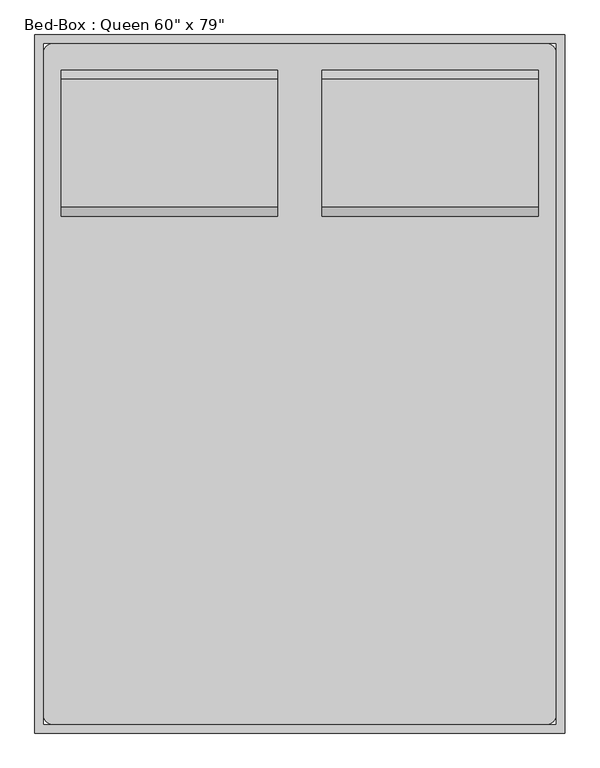
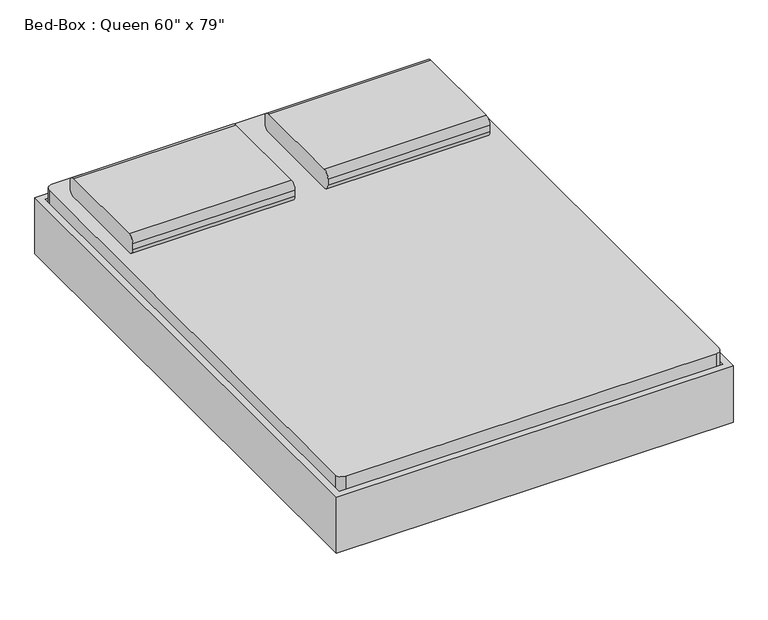
"""IFC4 building model written with IfcOpenShell, lengths in millimetres: furniture geometry."""

from ifc_helpers import new_model, si_unit, point, frame, frame_2d, origin, place, context, project, spatial, polyline, circle_curve, trimmed, segment, composite_curve, outline, extrude, source, transform, mapped, element, save
from ifc_brep_helpers import plane_surface, cylinder_surface, revolved_surface, advanced_brep


def furniture_0315470b(model_context):
    return source(origin(), model_context, "Body", "SolidModel", [
        advanced_brep(
        [(-397.447541, -932.9295082, 196.85), (-397.447541, -932.9295082, 177.8), (-397.447541, -1009.1295082, 177.8), (-397.447541, -1009.1295082, 196.85), (-334.5113525, -932.9295082, 196.85), (-346.647541, -932.9295082, 177.8), (-346.647541, -1009.1295082, 177.8), (-334.5113525, -1009.1295082, 196.85), (-253.3115092, -932.9295082, 22.716374), (-270.5766725, -932.9295082, 14.6654962), (-270.5766725, -1009.1295082, 14.6654962), (-253.3115092, -1009.1295082, 22.716374), (-247.5564547, -932.9295082, 0.0), (-247.5564547, -932.9295082, 19.05), (-247.5564547, -1009.1295082, 0.0), (-247.5564547, -1009.1295082, 19.05), (-168.9439489, -932.9295082, 19.05), (-168.9439489, -932.9295082, 0.0), (-168.9439489, -1009.1295082, 0.0), (-168.9439489, -1009.1295082, 19.05), (-156.2439489, -932.9295082, 3.4029547), (-165.7689489, -932.9295082, 19.9007387), (-156.2439489, -1009.1295082, 3.4029547), (-165.7689489, -1009.1295082, 19.9007387), (-101.2513357, -932.9295082, 57.15), (-96.1469036, -932.9295082, 38.1), (-96.1469036, -1009.1295082, 38.1), (-101.2513357, -1009.1295082, 57.15), (779.5562537, -932.9295082, 57.15), (774.4518216, -932.9295082, 38.1), (774.4518216, -1009.1295082, 38.1), (779.5562537, -1009.1295082, 57.15), (844.0738669, -932.9295082, 19.9007387), (834.5488669, -932.9295082, 3.4029547), (834.5488669, -1009.1295082, 3.4029547), (844.0738669, -1009.1295082, 19.9007387), (847.2488669, -932.9295082, 0.0), (847.2488669, -932.9295082, 19.05), (847.2488669, -1009.1295082, 0.0), (847.2488669, -1009.1295082, 19.05), (925.8613728, -932.9295082, 19.05), (925.8613728, -932.9295082, 0.0), (925.8613728, -1009.1295082, 0.0), (925.8613728, -1009.1295082, 19.05), (948.8815906, -932.9295082, 14.6654962), (931.6164272, -932.9295082, 22.716374), (948.8815906, -1009.1295082, 14.6654962), (931.6164272, -1009.1295082, 22.716374), (1012.8162705, -932.9295082, 196.85), (1024.952459, -932.9295082, 177.8), (1024.952459, -1009.1295082, 177.8), (1012.8162705, -1009.1295082, 196.85), (1075.752459, -932.9295082, 196.85), (1075.752459, -1009.1295082, 196.85), (1075.752459, -1009.1295082, 177.8), (1075.752459, -932.9295082, 177.8)],
        [
            (0, 1),
            (1, 2),
            (2, 3),
            (3, 0),
            (0, 4),
            (4, 5),
            (5, 1),
            (5, 6),
            (6, 2),
            (6, 7),
            (7, 3),
            (7, 4),
            (4, 8),
            (8, 9),
            (9, 5),
            (9, 10),
            (10, 6),
            (10, 11),
            (11, 7),
            (11, 8),
            (12, 9, circle_curve(frame((-247.5564547, -932.9295082, 25.4), z_axis=(0.0, 1.0, 0.0), x_axis=(-0.906307787036663, 0.0, -0.4226182617406713)), 25.4)),
            (8, 13, circle_curve(frame((-247.5564547, -932.9295082, 25.4), z_axis=(0.0, -1.0, 0.0), x_axis=(-0.906307787036663, 0.0, -0.4226182617406713)), 6.35)),
            (13, 12),
            (14, 10, circle_curve(frame((-247.5564547, -1009.1295082, 25.4), z_axis=(0.0, 1.0, 0.0), x_axis=(-0.906307787036663, 0.0, -0.4226182617406713)), 25.4)),
            (12, 14),
            (15, 11, circle_curve(frame((-247.5564547, -1009.1295082, 25.4), z_axis=(0.0, 1.0, 0.0), x_axis=(-0.906307787036663, 0.0, -0.4226182617406713)), 6.35)),
            (14, 15),
            (15, 13),
            (13, 16),
            (16, 17),
            (17, 12),
            (17, 18),
            (18, 14),
            (18, 19),
            (19, 15),
            (19, 16),
            (20, 17, circle_curve(frame((-168.9439489, -932.9295082, 25.4), z_axis=(0.0, 1.0, 0.0), x_axis=(0.0, 0.0, -1.0)), 25.4)),
            (16, 21, circle_curve(frame((-168.9439489, -932.9295082, 25.4), z_axis=(0.0, -1.0, 0.0), x_axis=(0.0, 0.0, -1.0)), 6.35)),
            (21, 20),
            (22, 18, circle_curve(frame((-168.9439489, -1009.1295082, 25.4), z_axis=(0.0, 1.0, 0.0), x_axis=(0.0, 0.0, -1.0)), 25.4)),
            (20, 22),
            (23, 19, circle_curve(frame((-168.9439489, -1009.1295082, 25.4), z_axis=(0.0, 1.0, 0.0), x_axis=(0.0, 0.0, -1.0)), 6.35)),
            (22, 23),
            (23, 21),
            (21, 24),
            (24, 25),
            (25, 20),
            (25, 26),
            (26, 22),
            (26, 27),
            (27, 23),
            (27, 24),
            (24, 28),
            (28, 29),
            (29, 25),
            (29, 30),
            (30, 26),
            (30, 31),
            (31, 27),
            (31, 28),
            (28, 32),
            (32, 33),
            (33, 29),
            (33, 34),
            (34, 30),
            (34, 35),
            (35, 31),
            (35, 32),
            (36, 33, circle_curve(frame((847.2488669, -932.9295082, 25.4), z_axis=(0.0, 1.0, 0.0), x_axis=(-0.5000000000000479, 0.0, -0.866025403784411)), 25.4)),
            (32, 37, circle_curve(frame((847.2488669, -932.9295082, 25.4), z_axis=(0.0, -1.0, 0.0), x_axis=(-0.5000000000000479, 0.0, -0.866025403784411)), 6.35)),
            (37, 36),
            (38, 34, circle_curve(frame((847.2488669, -1009.1295082, 25.4), z_axis=(0.0, 1.0, 0.0), x_axis=(-0.5000000000000479, 0.0, -0.866025403784411)), 25.4)),
            (36, 38),
            (39, 35, circle_curve(frame((847.2488669, -1009.1295082, 25.4), z_axis=(0.0, 1.0, 0.0), x_axis=(-0.5000000000000479, 0.0, -0.866025403784411)), 6.35)),
            (38, 39),
            (39, 37),
            (37, 40),
            (40, 41),
            (41, 36),
            (41, 42),
            (42, 38),
            (42, 43),
            (43, 39),
            (43, 40),
            (44, 41, circle_curve(frame((925.8613728, -932.9295082, 25.4), z_axis=(0.0, 1.0, 0.0), x_axis=(0.0, 0.0, -1.0)), 25.4)),
            (40, 45, circle_curve(frame((925.8613728, -932.9295082, 25.4), z_axis=(0.0, -1.0, 0.0), x_axis=(0.0, 0.0, -1.0)), 6.35)),
            (45, 44),
            (46, 42, circle_curve(frame((925.8613728, -1009.1295082, 25.4), z_axis=(0.0, 1.0, 0.0), x_axis=(0.0, 0.0, -1.0)), 25.4)),
            (44, 46),
            (47, 43, circle_curve(frame((925.8613728, -1009.1295082, 25.4), z_axis=(0.0, 1.0, 0.0), x_axis=(0.0, 0.0, -1.0)), 6.35)),
            (46, 47),
            (47, 45),
            (45, 48),
            (48, 49),
            (49, 44),
            (49, 50),
            (50, 46),
            (50, 51),
            (51, 47),
            (51, 48),
            (52, 53),
            (53, 54),
            (54, 55),
            (55, 52),
            (48, 52),
            (55, 49),
            (54, 50),
            (53, 51),
        ],
        [
            plane_surface(frame((-397.447541, -1237.7295082, -127.5947323), z_axis=(-1.0, 0.0, 0.0), x_axis=(0.0, 1.0, 0.0))),
            plane_surface(frame((-397.447541, -932.9295082, 196.85), z_axis=(0.0, 1.0, 0.0), x_axis=(1.0, 0.0, 0.0))),
            plane_surface(frame((-397.447541, -932.9295082, 177.8), z_axis=(0.0, 0.0, -1.0), x_axis=(1.0, 0.0, 0.0))),
            plane_surface(frame((-397.447541, -1009.1295082, 177.8), z_axis=(0.0, -1.0, 0.0), x_axis=(1.0, 0.0, 0.0))),
            plane_surface(frame((-397.447541, -1009.1295082, 196.85), z_axis=(0.0, 0.0, 1.0), x_axis=(1.0, 0.0, 0.0))),
            plane_surface(frame((-334.5113525, -932.9295082, 196.85), z_axis=(0.0, 1.0, 0.0), x_axis=(0.4226182617406707, 0.0, -0.9063077870366634))),
            plane_surface(frame((-346.647541, -932.9295082, 177.8), z_axis=(-0.9063077870366635, 0.0, -0.4226182617406707), x_axis=(0.4226182617406707, 0.0, -0.9063077870366635))),
            plane_surface(frame((-346.647541, -1009.1295082, 177.8), z_axis=(0.0, -1.0, 0.0), x_axis=(0.422618261740671, 0.0, -0.9063077870366633))),
            plane_surface(frame((-334.5113525, -1009.1295082, 196.85), z_axis=(0.9063077870366633, 0.0, 0.42261826174067113), x_axis=(0.42261826174067113, 0.0, -0.9063077870366633))),
            plane_surface(frame((-247.5564547, -932.9295082, 25.4), z_axis=(0.0, 1.0, 0.0), x_axis=(-0.906307787036663, 0.0, -0.4226182617406713))),
            cylinder_surface(frame((-247.5564547, -1237.7295082, 25.4), z_axis=(0.0, -1.0, 0.0), x_axis=(-0.906307787036663, 0.0, -0.4226182617406713)), 25.4),
            plane_surface(frame((-247.5564547, -1009.1295082, 25.4), z_axis=(0.0, -1.0, 0.0), x_axis=(-0.906307787036663, 0.0, -0.4226182617406713))),
            revolved_surface(polyline([(-253.3115091476828, -1009.1295082, 22.716374037946736), (-253.3115091476828, -932.9295082, 22.716374037946736)]), (-247.5564547, -1237.7295082, 25.4), (0.0, -1.0, 0.0)),
            plane_surface(frame((-247.5564547, -932.9295082, 19.05), z_axis=(0.0, 1.0, 0.0), x_axis=(1.0, 0.0, 0.0))),
            plane_surface(frame((-247.5564547, -932.9295082, 0.0), z_axis=(0.0, 0.0, -1.0), x_axis=(1.0, 0.0, 0.0))),
            plane_surface(frame((-247.5564547, -1009.1295082, 0.0), z_axis=(0.0, -1.0, 0.0), x_axis=(1.0, 0.0, 0.0))),
            plane_surface(frame((-247.5564547, -1009.1295082, 19.05), z_axis=(0.0, 0.0, 1.0), x_axis=(1.0, 0.0, 0.0))),
            plane_surface(frame((-168.9439489, -932.9295082, 25.4), z_axis=(0.0, 1.0, 0.0), x_axis=(0.0, 0.0, -1.0))),
            cylinder_surface(frame((-168.9439489, -1237.7295082, 25.4), z_axis=(0.0, -1.0, 0.0), x_axis=(0.0, 0.0, -1.0)), 25.4),
            plane_surface(frame((-168.9439489, -1009.1295082, 25.4), z_axis=(0.0, -1.0, 0.0), x_axis=(0.0, 0.0, -1.0))),
            revolved_surface(polyline([(-168.9439489, -1009.1295082, 19.049999999999997), (-168.9439489, -932.9295082, 19.049999999999997)]), (-168.9439489, -1237.7295082, 25.4), (0.0, -1.0, 0.0)),
            plane_surface(frame((-165.7689489, -932.9295082, 19.9007387), z_axis=(0.0, 1.0, 0.0), x_axis=(0.8660254037844788, 0.0, 0.4999999999999306))),
            plane_surface(frame((-156.2439489, -932.9295082, 3.4029547), z_axis=(0.49999999999993017, 0.0, -0.866025403784479), x_axis=(0.866025403784479, 0.0, 0.49999999999993017))),
            plane_surface(frame((-156.2439489, -1009.1295082, 3.4029547), z_axis=(0.0, -1.0, 0.0), x_axis=(0.8660254037844785, 0.0, 0.49999999999993106))),
            plane_surface(frame((-165.7689489, -1009.1295082, 19.9007387), z_axis=(-0.4999999999999309, 0.0, 0.8660254037844786), x_axis=(0.8660254037844786, 0.0, 0.4999999999999309))),
            plane_surface(frame((-101.2513357, -932.9295082, 57.15), z_axis=(0.0, 1.0, 0.0), x_axis=(1.0, 0.0, 0.0))),
            plane_surface(frame((-96.1469036, -932.9295082, 38.1), z_axis=(0.0, 0.0, -1.0), x_axis=(1.0, 0.0, 0.0))),
            plane_surface(frame((-96.1469036, -1009.1295082, 38.1), z_axis=(0.0, -1.0, 0.0), x_axis=(1.0, 0.0, 0.0))),
            plane_surface(frame((-101.2513357, -1009.1295082, 57.15), z_axis=(0.0, 0.0, 1.0), x_axis=(1.0, 0.0, 0.0))),
            plane_surface(frame((779.5562537, -932.9295082, 57.15), z_axis=(0.0, 1.0000000000000002, 0.0), x_axis=(0.8660254037844106, 0.0, -0.5000000000000487))),
            plane_surface(frame((774.4518216, -932.9295082, 38.1), z_axis=(-0.5000000000000477, 0.0, -0.8660254037844112), x_axis=(0.8660254037844112, 0.0, -0.5000000000000477))),
            plane_surface(frame((774.4518216, -1009.1295082, 38.1), z_axis=(0.0, -1.0000000000000002, 0.0), x_axis=(0.8660254037844105, 0.0, -0.500000000000049))),
            plane_surface(frame((779.5562537, -1009.1295082, 57.15), z_axis=(0.5000000000000498, 0.0, 0.8660254037844098), x_axis=(0.8660254037844098, 0.0, -0.5000000000000498))),
            plane_surface(frame((847.2488669, -932.9295082, 25.4), z_axis=(0.0, 1.0000000000000002, 0.0), x_axis=(-0.500000000000048, 0.0, -0.8660254037844111))),
            cylinder_surface(frame((847.2488669, -1237.7295082, 25.4), z_axis=(0.0, -1.0, 0.0), x_axis=(-0.5000000000000479, 0.0, -0.866025403784411)), 25.4),
            plane_surface(frame((847.2488669, -1009.1295082, 25.4), z_axis=(0.0, -1.0000000000000002, 0.0), x_axis=(-0.500000000000048, 0.0, -0.8660254037844111))),
            revolved_surface(polyline([(844.0738668999998, -1009.1295082, 19.90073868596899), (844.0738668999998, -932.9295082, 19.90073868596899)]), (847.2488669, -1237.7295082, 25.4), (0.0, -1.0, 0.0)),
            plane_surface(frame((847.2488669, -932.9295082, 19.05), z_axis=(0.0, 1.0, 0.0), x_axis=(1.0, 0.0, 0.0))),
            plane_surface(frame((847.2488669, -932.9295082, 0.0), z_axis=(0.0, 0.0, -1.0), x_axis=(1.0, 0.0, 0.0))),
            plane_surface(frame((847.2488669, -1009.1295082, 0.0), z_axis=(0.0, -1.0, 0.0), x_axis=(1.0, 0.0, 0.0))),
            plane_surface(frame((847.2488669, -1009.1295082, 19.05), z_axis=(0.0, 0.0, 1.0), x_axis=(1.0, 0.0, 0.0))),
            plane_surface(frame((925.8613728, -932.9295082, 25.4), z_axis=(0.0, 1.0, 0.0), x_axis=(0.0, 0.0, -1.0))),
            cylinder_surface(frame((925.8613728, -1237.7295082, 25.4), z_axis=(0.0, -1.0, 0.0), x_axis=(0.0, 0.0, -1.0)), 25.4),
            plane_surface(frame((925.8613728, -1009.1295082, 25.4), z_axis=(0.0, -1.0, 0.0), x_axis=(0.0, 0.0, -1.0))),
            revolved_surface(polyline([(925.8613728, -1009.1295082, 19.049999999999997), (925.8613728, -932.9295082, 19.049999999999997)]), (925.8613728, -1237.7295082, 25.4), (0.0, -1.0, 0.0)),
            plane_surface(frame((931.6164272, -932.9295082, 22.716374), z_axis=(0.0, 1.0, 0.0), x_axis=(0.4226182617405411, 0.0, 0.9063077870367238))),
            plane_surface(frame((948.8815906, -932.9295082, 14.6654962), z_axis=(0.9063077870367237, 0.0, -0.4226182617405414), x_axis=(0.4226182617405414, 0.0, 0.9063077870367237))),
            plane_surface(frame((948.8815906, -1009.1295082, 14.6654962), z_axis=(0.0, -1.0, 0.0), x_axis=(0.42261826174054123, 0.0, 0.9063077870367238))),
            plane_surface(frame((931.6164272, -1009.1295082, 22.716374), z_axis=(-0.9063077870367237, 0.0, 0.4226182617405414), x_axis=(0.4226182617405414, 0.0, 0.9063077870367237))),
            plane_surface(frame((1075.752459, -1237.7295082, -127.5947323), z_axis=(1.0, 0.0, 0.0), x_axis=(0.0, 1.0, 0.0))),
            plane_surface(frame((1012.8162705, -932.9295082, 196.85), z_axis=(0.0, 1.0, 0.0), x_axis=(1.0, 0.0, 0.0))),
            plane_surface(frame((1024.952459, -932.9295082, 177.8), z_axis=(0.0, 0.0, -1.0), x_axis=(1.0, 0.0, 0.0))),
            plane_surface(frame((1024.952459, -1009.1295082, 177.8), z_axis=(0.0, -1.0, 0.0), x_axis=(1.0, 0.0, 0.0))),
            plane_surface(frame((1012.8162705, -1009.1295082, 196.85), z_axis=(0.0, 0.0, 1.0), x_axis=(1.0, 0.0, 0.0))),
        ],
        [
            (0, [[1, 2, 3, 4]]),
            (1, [[-1, 5, 6, 7]]),
            (2, [[-2, -7, 8, 9]]),
            (3, [[-3, -9, 10, 11]]),
            (4, [[-4, -11, 12, -5]]),
            (5, [[-6, 13, 14, 15]]),
            (6, [[-8, -15, 16, 17]]),
            (7, [[-10, -17, 18, 19]]),
            (8, [[-12, -19, 20, -13]]),
            (9, [[21, -14, 22, 23]]),
            (10, [[24, -16, -21, 25]]),
            (11, [[26, -18, -24, 27]]),
            (12, [[-22, -20, -26, 28]]),
            (13, [[-23, 29, 30, 31]]),
            (14, [[-25, -31, 32, 33]]),
            (15, [[-27, -33, 34, 35]]),
            (16, [[-28, -35, 36, -29]]),
            (17, [[37, -30, 38, 39]]),
            (18, [[40, -32, -37, 41]]),
            (19, [[42, -34, -40, 43]]),
            (20, [[-38, -36, -42, 44]]),
            (21, [[-39, 45, 46, 47]]),
            (22, [[-41, -47, 48, 49]]),
            (23, [[-43, -49, 50, 51]]),
            (24, [[-44, -51, 52, -45]]),
            (25, [[-46, 53, 54, 55]]),
            (26, [[-48, -55, 56, 57]]),
            (27, [[-50, -57, 58, 59]]),
            (28, [[-52, -59, 60, -53]]),
            (29, [[-54, 61, 62, 63]]),
            (30, [[-56, -63, 64, 65]]),
            (31, [[-58, -65, 66, 67]]),
            (32, [[-60, -67, 68, -61]]),
            (33, [[69, -62, 70, 71]]),
            (34, [[72, -64, -69, 73]]),
            (35, [[74, -66, -72, 75]]),
            (36, [[-70, -68, -74, 76]]),
            (37, [[-71, 77, 78, 79]]),
            (38, [[-73, -79, 80, 81]]),
            (39, [[-75, -81, 82, 83]]),
            (40, [[-76, -83, 84, -77]]),
            (41, [[85, -78, 86, 87]]),
            (42, [[88, -80, -85, 89]]),
            (43, [[90, -82, -88, 91]]),
            (44, [[-86, -84, -90, 92]]),
            (45, [[-87, 93, 94, 95]]),
            (46, [[-89, -95, 96, 97]]),
            (47, [[-91, -97, 98, 99]]),
            (48, [[-92, -99, 100, -93]]),
            (49, [[101, 102, 103, 104]]),
            (50, [[-94, 105, -104, 106]]),
            (51, [[-96, -106, -103, 107]]),
            (52, [[-98, -107, -102, 108]]),
            (53, [[-100, -108, -101, -105]]),
        ],
    ),
        extrude(outline(composite_curve([segment(polyline([(-372.047541, 743.4704918), (1050.352459, 743.4704918)]), True, "CONTINUOUS"), segment(trimmed(circle_curve(frame_2d((1050.352459, 718.0704918)), 25.4), [point((1050.352459, 743.4704918))], [point((1075.752459, 718.0704918))], False, "CARTESIAN"), True, "CONTINUOUS"), segment(polyline([(1075.752459, 718.0704918), (1075.752459, -1186.9295082)]), True, "CONTINUOUS"), segment(trimmed(circle_curve(frame_2d((1050.352459, -1186.9295082)), 25.4), [point((1075.752459, -1186.9295082))], [point((1050.352459, -1212.3295082))], False, "CARTESIAN"), True, "CONTINUOUS"), segment(polyline([(1050.352459, -1212.3295082), (-372.047541, -1212.3295082)]), True, "CONTINUOUS"), segment(trimmed(circle_curve(frame_2d((-372.047541, -1186.9295082)), 25.4), [point((-372.047541, -1212.3295082))], [point((-397.447541, -1186.9295082))], False, "CARTESIAN"), True, "CONTINUOUS"), segment(polyline([(-397.447541, -1186.9295082), (-397.447541, 718.0704918)]), True, "CONTINUOUS"), segment(trimmed(circle_curve(frame_2d((-372.047541, 718.0704918)), 25.4), [point((-397.447541, 718.0704918))], [point((-372.047541, 743.4704918))], False, "CARTESIAN"), True, "CONTINUOUS")], self_intersect=False)), frame((0.0, 0.0, 203.2), z_axis=(0.0, 0.0, 1.0), x_axis=(1.0, 0.0, 0.0)), (0.0, 0.0, 1.0), 203.2),
        advanced_brep(
        [(-397.1231784, 514.8704918, 177.8), (-397.1231784, 438.6704918, 177.8), (-397.1231784, 438.6704918, 196.85), (-397.1231784, 514.8704918, 196.85), (-346.3231784, 514.8704918, 177.8), (-346.3231784, 438.6704918, 177.8), (-334.1869899, 438.6704918, 196.85), (-334.1869899, 514.8704918, 196.85), (-270.2523099, 514.8704918, 14.6654962), (-270.2523099, 438.6704918, 14.6654962), (-252.9871466, 438.6704918, 22.716374), (-252.9871466, 514.8704918, 22.716374), (-247.2320921, 438.6704918, 0.0), (-247.2320921, 514.8704918, 0.0), (-247.2320921, 438.6704918, 19.05), (-247.2320921, 514.8704918, 19.05), (-168.6195862, 514.8704918, 0.0), (-168.6195862, 438.6704918, 0.0), (-168.6195862, 438.6704918, 19.05), (-168.6195862, 514.8704918, 19.05), (-155.9195862, 438.6704918, 3.4029547), (-155.9195862, 514.8704918, 3.4029547), (-165.4445862, 438.6704918, 19.9007387), (-165.4445862, 514.8704918, 19.9007387), (-95.822541, 514.8704918, 38.1), (-95.822541, 438.6704918, 38.1), (-100.9269731, 438.6704918, 57.15), (-100.9269731, 514.8704918, 57.15), (774.4518216, 514.8704918, 38.1), (774.4518216, 438.6704918, 38.1), (779.5562537, 438.6704918, 57.15), (779.5562537, 514.8704918, 57.15), (834.5488669, 514.8704918, 3.4029547), (834.5488669, 438.6704918, 3.4029547), (844.0738669, 438.6704918, 19.9007387), (844.0738669, 514.8704918, 19.9007387), (847.2488669, 438.6704918, 0.0), (847.2488669, 514.8704918, 0.0), (847.2488669, 438.6704918, 19.05), (847.2488669, 514.8704918, 19.05), (925.8613728, 514.8704918, 0.0), (925.8613728, 438.6704918, 0.0), (925.8613728, 438.6704918, 19.05), (925.8613728, 514.8704918, 19.05), (948.8815906, 438.6704918, 14.6654962), (948.8815906, 514.8704918, 14.6654962), (931.6164272, 438.6704918, 22.716374), (931.6164272, 514.8704918, 22.716374), (1024.952459, 514.8704918, 177.8), (1024.952459, 438.6704918, 177.8), (1012.8162705, 438.6704918, 196.85), (1012.8162705, 514.8704918, 196.85), (1075.752459, 514.8704918, 177.8), (1075.752459, 514.8704918, 196.85), (1075.752459, 438.6704918, 196.85), (1075.752459, 438.6704918, 177.8)],
        [
            (0, 1),
            (1, 2),
            (2, 3),
            (3, 0),
            (0, 4),
            (4, 5),
            (5, 1),
            (5, 6),
            (6, 2),
            (6, 7),
            (7, 3),
            (7, 4),
            (4, 8),
            (8, 9),
            (9, 5),
            (9, 10),
            (10, 6),
            (10, 11),
            (11, 7),
            (11, 8),
            (12, 9, circle_curve(frame((-247.2320921, 438.6704918, 25.4), z_axis=(0.0, 1.0, 0.0), x_axis=(-0.9063077870366486, 0.0, -0.42261826174070233)), 25.4)),
            (8, 13, circle_curve(frame((-247.2320921, 514.8704918, 25.4), z_axis=(0.0, -1.0, 0.0), x_axis=(-0.9063077870366486, 0.0, -0.42261826174070233)), 25.4)),
            (13, 12),
            (14, 10, circle_curve(frame((-247.2320921, 438.6704918, 25.4), z_axis=(0.0, 1.0, 0.0), x_axis=(-0.9063077870366486, 0.0, -0.42261826174070233)), 6.35)),
            (12, 14),
            (15, 11, circle_curve(frame((-247.2320921, 514.8704918, 25.4), z_axis=(0.0, 1.0, 0.0), x_axis=(-0.9063077870366486, 0.0, -0.42261826174070233)), 6.35)),
            (14, 15),
            (15, 13),
            (13, 16),
            (16, 17),
            (17, 12),
            (17, 18),
            (18, 14),
            (18, 19),
            (19, 15),
            (19, 16),
            (20, 17, circle_curve(frame((-168.6195862, 438.6704918, 25.4), z_axis=(0.0, 1.0, 0.0), x_axis=(0.0, 0.0, -1.0)), 25.4)),
            (16, 21, circle_curve(frame((-168.6195862, 514.8704918, 25.4), z_axis=(0.0, -1.0, 0.0), x_axis=(0.0, 0.0, -1.0)), 25.4)),
            (21, 20),
            (22, 18, circle_curve(frame((-168.6195862, 438.6704918, 25.4), z_axis=(0.0, 1.0, 0.0), x_axis=(0.0, 0.0, -1.0)), 6.35)),
            (20, 22),
            (23, 19, circle_curve(frame((-168.6195862, 514.8704918, 25.4), z_axis=(0.0, 1.0, 0.0), x_axis=(0.0, 0.0, -1.0)), 6.35)),
            (22, 23),
            (23, 21),
            (21, 24),
            (24, 25),
            (25, 20),
            (25, 26),
            (26, 22),
            (26, 27),
            (27, 23),
            (27, 24),
            (24, 28),
            (28, 29),
            (29, 25),
            (29, 30),
            (30, 26),
            (30, 31),
            (31, 27),
            (31, 28),
            (28, 32),
            (32, 33),
            (33, 29),
            (33, 34),
            (34, 30),
            (34, 35),
            (35, 31),
            (35, 32),
            (36, 33, circle_curve(frame((847.2488669, 438.6704918, 25.4), z_axis=(0.0, 1.0, 0.0), x_axis=(-0.5000000000000463, 0.0, -0.8660254037844118)), 25.4)),
            (32, 37, circle_curve(frame((847.2488669, 514.8704918, 25.4), z_axis=(0.0, -1.0, 0.0), x_axis=(-0.5000000000000463, 0.0, -0.8660254037844118)), 25.4)),
            (37, 36),
            (38, 34, circle_curve(frame((847.2488669, 438.6704918, 25.4), z_axis=(0.0, 1.0, 0.0), x_axis=(-0.5000000000000463, 0.0, -0.8660254037844118)), 6.35)),
            (36, 38),
            (39, 35, circle_curve(frame((847.2488669, 514.8704918, 25.4), z_axis=(0.0, 1.0, 0.0), x_axis=(-0.5000000000000463, 0.0, -0.8660254037844118)), 6.35)),
            (38, 39),
            (39, 37),
            (37, 40),
            (40, 41),
            (41, 36),
            (41, 42),
            (42, 38),
            (42, 43),
            (43, 39),
            (43, 40),
            (44, 41, circle_curve(frame((925.8613728, 438.6704918, 25.4), z_axis=(0.0, 1.0, 0.0), x_axis=(0.0, 0.0, -1.0)), 25.4)),
            (40, 45, circle_curve(frame((925.8613728, 514.8704918, 25.4), z_axis=(0.0, -1.0, 0.0), x_axis=(0.0, 0.0, -1.0)), 25.4)),
            (45, 44),
            (46, 42, circle_curve(frame((925.8613728, 438.6704918, 25.4), z_axis=(0.0, 1.0, 0.0), x_axis=(0.0, 0.0, -1.0)), 6.35)),
            (44, 46),
            (47, 43, circle_curve(frame((925.8613728, 514.8704918, 25.4), z_axis=(0.0, 1.0, 0.0), x_axis=(0.0, 0.0, -1.0)), 6.35)),
            (46, 47),
            (47, 45),
            (45, 48),
            (48, 49),
            (49, 44),
            (49, 50),
            (50, 46),
            (50, 51),
            (51, 47),
            (51, 48),
            (52, 53),
            (53, 54),
            (54, 55),
            (55, 52),
            (48, 52),
            (55, 49),
            (54, 50),
            (53, 51),
        ],
        [
            plane_surface(frame((-397.1231784, 768.8704918, -152.9490627), z_axis=(-1.0, 0.0, 0.0), x_axis=(0.0, 1.0, 0.0))),
            plane_surface(frame((-397.1231784, 514.8704918, 177.8), z_axis=(0.0, 0.0, -1.0), x_axis=(1.0, 0.0, 0.0))),
            plane_surface(frame((-397.1231784, 438.6704918, 177.8), z_axis=(0.0, -1.0, 0.0), x_axis=(1.0, 0.0, 0.0))),
            plane_surface(frame((-397.1231784, 438.6704918, 196.85), z_axis=(0.0, 0.0, 1.0), x_axis=(1.0, 0.0, 0.0))),
            plane_surface(frame((-397.1231784, 514.8704918, 196.85), z_axis=(0.0, 1.0, 0.0), x_axis=(1.0, 0.0, 0.0))),
            plane_surface(frame((-346.3231784, 514.8704918, 177.8), z_axis=(-0.9063077870366485, 0.0, -0.4226182617407027), x_axis=(0.4226182617407027, 0.0, -0.9063077870366485))),
            plane_surface(frame((-346.3231784, 438.6704918, 177.8), z_axis=(0.0, -1.0, 0.0), x_axis=(0.4226182617407025, 0.0, -0.9063077870366486))),
            plane_surface(frame((-334.1869899, 438.6704918, 196.85), z_axis=(0.9063077870366484, 0.0, 0.4226182617407028), x_axis=(0.4226182617407028, 0.0, -0.9063077870366484))),
            plane_surface(frame((-334.1869899, 514.8704918, 196.85), z_axis=(0.0, 1.0, 0.0), x_axis=(0.42261826174070277, 0.0, -0.9063077870366485))),
            cylinder_surface(frame((-247.2320921, 768.8704918, 25.4), z_axis=(0.0, -1.0, 0.0), x_axis=(-0.9063077870366486, 0.0, -0.42261826174070233)), 25.4),
            plane_surface(frame((-247.2320921, 438.6704918, 25.4), z_axis=(0.0, -1.0, 0.0), x_axis=(-0.9063077870366486, 0.0, -0.42261826174070233))),
            revolved_surface(polyline([(-252.9871465476827, 438.6704918, 22.71637403794654), (-252.9871465476827, 514.8704918, 22.71637403794654)]), (-247.2320921, 768.8704918, 25.4), (0.0, -1.0, 0.0)),
            plane_surface(frame((-247.2320921, 514.8704918, 25.4), z_axis=(0.0, 1.0, 0.0), x_axis=(-0.9063077870366486, 0.0, -0.42261826174070233))),
            plane_surface(frame((-247.2320921, 514.8704918, 0.0), z_axis=(0.0, 0.0, -1.0), x_axis=(1.0, 0.0, 0.0))),
            plane_surface(frame((-247.2320921, 438.6704918, 0.0), z_axis=(0.0, -1.0, 0.0), x_axis=(1.0, 0.0, 0.0))),
            plane_surface(frame((-247.2320921, 438.6704918, 19.05), z_axis=(0.0, 0.0, 1.0), x_axis=(1.0, 0.0, 0.0))),
            plane_surface(frame((-247.2320921, 514.8704918, 19.05), z_axis=(0.0, 1.0, 0.0), x_axis=(1.0, 0.0, 0.0))),
            cylinder_surface(frame((-168.6195862, 768.8704918, 25.4), z_axis=(0.0, -1.0, 0.0), x_axis=(0.0, 0.0, -1.0)), 25.4),
            plane_surface(frame((-168.6195862, 438.6704918, 25.4), z_axis=(0.0, -1.0, 0.0), x_axis=(0.0, 0.0, -1.0))),
            revolved_surface(polyline([(-168.6195862, 438.6704918, 19.049999999999997), (-168.6195862, 514.8704918, 19.049999999999997)]), (-168.6195862, 768.8704918, 25.4), (0.0, -1.0, 0.0)),
            plane_surface(frame((-168.6195862, 514.8704918, 25.4), z_axis=(0.0, 1.0, 0.0), x_axis=(0.0, 0.0, -1.0))),
            plane_surface(frame((-155.9195862, 514.8704918, 3.4029547), z_axis=(0.49999999999988004, 0.0, -0.866025403784508), x_axis=(0.866025403784508, 0.0, 0.49999999999988004))),
            plane_surface(frame((-155.9195862, 438.6704918, 3.4029547), z_axis=(0.0, -1.0, 0.0), x_axis=(0.8660254037845078, 0.0, 0.49999999999988026))),
            plane_surface(frame((-165.4445862, 438.6704918, 19.9007387), z_axis=(-0.4999999999998799, 0.0, 0.866025403784508), x_axis=(0.866025403784508, 0.0, 0.4999999999998799))),
            plane_surface(frame((-165.4445862, 514.8704918, 19.9007387), z_axis=(0.0, 1.0, 0.0), x_axis=(0.8660254037845075, 0.0, 0.49999999999988076))),
            plane_surface(frame((-95.822541, 514.8704918, 38.1), z_axis=(0.0, 0.0, -1.0), x_axis=(1.0, 0.0, 0.0))),
            plane_surface(frame((-95.822541, 438.6704918, 38.1), z_axis=(0.0, -1.0, 0.0), x_axis=(1.0, 0.0, 0.0))),
            plane_surface(frame((-100.9269731, 438.6704918, 57.15), z_axis=(0.0, 0.0, 1.0), x_axis=(1.0, 0.0, 0.0))),
            plane_surface(frame((-100.9269731, 514.8704918, 57.15), z_axis=(0.0, 1.0, 0.0), x_axis=(1.0, 0.0, 0.0))),
            plane_surface(frame((774.4518216, 514.8704918, 38.1), z_axis=(-0.5000000000000455, 0.0, -0.8660254037844125), x_axis=(0.8660254037844125, 0.0, -0.5000000000000455))),
            plane_surface(frame((774.4518216, 438.6704918, 38.1), z_axis=(0.0, -1.0, 0.0), x_axis=(0.866025403784412, 0.0, -0.5000000000000463))),
            plane_surface(frame((779.5562537, 438.6704918, 57.15), z_axis=(0.5000000000000466, 0.0, 0.8660254037844117), x_axis=(0.8660254037844117, 0.0, -0.5000000000000466))),
            plane_surface(frame((779.5562537, 514.8704918, 57.15), z_axis=(0.0, 1.0, 0.0), x_axis=(0.8660254037844115, 0.0, -0.5000000000000471))),
            cylinder_surface(frame((847.2488669, 768.8704918, 25.4), z_axis=(0.0, -1.0, 0.0), x_axis=(-0.5000000000000463, 0.0, -0.8660254037844118)), 25.4),
            plane_surface(frame((847.2488669, 438.6704918, 25.4), z_axis=(0.0, -1.0000000000000002, 0.0), x_axis=(-0.5000000000000464, 0.0, -0.866025403784412))),
            revolved_surface(polyline([(844.0738668999998, 438.6704918, 19.90073868596898), (844.0738668999998, 514.8704918, 19.90073868596898)]), (847.2488669, 768.8704918, 25.4), (0.0, -1.0, 0.0)),
            plane_surface(frame((847.2488669, 514.8704918, 25.4), z_axis=(0.0, 1.0000000000000002, 0.0), x_axis=(-0.5000000000000464, 0.0, -0.866025403784412))),
            plane_surface(frame((847.2488669, 514.8704918, 0.0), z_axis=(0.0, 0.0, -1.0), x_axis=(1.0, 0.0, 0.0))),
            plane_surface(frame((847.2488669, 438.6704918, 0.0), z_axis=(0.0, -1.0, 0.0), x_axis=(1.0, 0.0, 0.0))),
            plane_surface(frame((847.2488669, 438.6704918, 19.05), z_axis=(0.0, 0.0, 1.0), x_axis=(1.0, 0.0, 0.0))),
            plane_surface(frame((847.2488669, 514.8704918, 19.05), z_axis=(0.0, 1.0, 0.0), x_axis=(1.0, 0.0, 0.0))),
            cylinder_surface(frame((925.8613728, 768.8704918, 25.4), z_axis=(0.0, -1.0, 0.0), x_axis=(0.0, 0.0, -1.0)), 25.4),
            plane_surface(frame((925.8613728, 438.6704918, 25.4), z_axis=(0.0, -1.0, 0.0), x_axis=(0.0, 0.0, -1.0))),
            revolved_surface(polyline([(925.8613728, 438.6704918, 19.049999999999997), (925.8613728, 514.8704918, 19.049999999999997)]), (925.8613728, 768.8704918, 25.4), (0.0, -1.0, 0.0)),
            plane_surface(frame((925.8613728, 514.8704918, 25.4), z_axis=(0.0, 1.0, 0.0), x_axis=(0.0, 0.0, -1.0))),
            plane_surface(frame((948.8815906, 514.8704918, 14.6654962), z_axis=(0.90630778703668, 0.0, -0.42261826174063505), x_axis=(0.42261826174063505, 0.0, 0.90630778703668))),
            plane_surface(frame((948.8815906, 438.6704918, 14.6654962), z_axis=(0.0, -1.0, 0.0), x_axis=(0.42261826174063566, 0.0, 0.9063077870366797))),
            plane_surface(frame((931.6164272, 438.6704918, 22.716374), z_axis=(-0.9063077870366801, 0.0, 0.42261826174063477), x_axis=(0.42261826174063477, 0.0, 0.9063077870366801))),
            plane_surface(frame((931.6164272, 514.8704918, 22.716374), z_axis=(0.0, 1.0, 0.0), x_axis=(0.4226182617406345, 0.0, 0.9063077870366802))),
            plane_surface(frame((1075.752459, 768.8704918, -152.9490627), z_axis=(1.0, 0.0, 0.0), x_axis=(0.0, 1.0, 0.0))),
            plane_surface(frame((1024.952459, 514.8704918, 177.8), z_axis=(0.0, 0.0, -1.0), x_axis=(1.0, 0.0, 0.0))),
            plane_surface(frame((1024.952459, 438.6704918, 177.8), z_axis=(0.0, -1.0, 0.0), x_axis=(1.0, 0.0, 0.0))),
            plane_surface(frame((1012.8162705, 438.6704918, 196.85), z_axis=(0.0, 0.0, 1.0), x_axis=(1.0, 0.0, 0.0))),
            plane_surface(frame((1012.8162705, 514.8704918, 196.85), z_axis=(0.0, 1.0, 0.0), x_axis=(1.0, 0.0, 0.0))),
        ],
        [
            (0, [[1, 2, 3, 4]]),
            (1, [[-1, 5, 6, 7]]),
            (2, [[-2, -7, 8, 9]]),
            (3, [[-3, -9, 10, 11]]),
            (4, [[-4, -11, 12, -5]]),
            (5, [[-6, 13, 14, 15]]),
            (6, [[-8, -15, 16, 17]]),
            (7, [[-10, -17, 18, 19]]),
            (8, [[-12, -19, 20, -13]]),
            (9, [[21, -14, 22, 23]]),
            (10, [[24, -16, -21, 25]]),
            (11, [[26, -18, -24, 27]]),
            (12, [[-22, -20, -26, 28]]),
            (13, [[-23, 29, 30, 31]]),
            (14, [[-25, -31, 32, 33]]),
            (15, [[-27, -33, 34, 35]]),
            (16, [[-28, -35, 36, -29]]),
            (17, [[37, -30, 38, 39]]),
            (18, [[40, -32, -37, 41]]),
            (19, [[42, -34, -40, 43]]),
            (20, [[-38, -36, -42, 44]]),
            (21, [[-39, 45, 46, 47]]),
            (22, [[-41, -47, 48, 49]]),
            (23, [[-43, -49, 50, 51]]),
            (24, [[-44, -51, 52, -45]]),
            (25, [[-46, 53, 54, 55]]),
            (26, [[-48, -55, 56, 57]]),
            (27, [[-50, -57, 58, 59]]),
            (28, [[-52, -59, 60, -53]]),
            (29, [[-54, 61, 62, 63]]),
            (30, [[-56, -63, 64, 65]]),
            (31, [[-58, -65, 66, 67]]),
            (32, [[-60, -67, 68, -61]]),
            (33, [[69, -62, 70, 71]]),
            (34, [[72, -64, -69, 73]]),
            (35, [[74, -66, -72, 75]]),
            (36, [[-70, -68, -74, 76]]),
            (37, [[-71, 77, 78, 79]]),
            (38, [[-73, -79, 80, 81]]),
            (39, [[-75, -81, 82, 83]]),
            (40, [[-76, -83, 84, -77]]),
            (41, [[85, -78, 86, 87]]),
            (42, [[88, -80, -85, 89]]),
            (43, [[90, -82, -88, 91]]),
            (44, [[-86, -84, -90, 92]]),
            (45, [[-87, 93, 94, 95]]),
            (46, [[-89, -95, 96, 97]]),
            (47, [[-91, -97, 98, 99]]),
            (48, [[-92, -99, 100, -93]]),
            (49, [[101, 102, 103, 104]]),
            (50, [[-94, 105, -104, 106]]),
            (51, [[-96, -106, -103, 107]]),
            (52, [[-98, -107, -102, 108]]),
            (53, [[-100, -108, -101, -105]]),
        ],
    ),
        extrude(outline(composite_curve([segment(polyline([(641.8704918, 406.4), (273.5704918, 406.4)]), True, "CONTINUOUS"), segment(trimmed(circle_curve(frame_2d((273.5704918, 431.8)), 25.4), [point((273.5704918, 406.4))], [point((248.1704918, 431.8))], False, "CARTESIAN"), True, "CONTINUOUS"), segment(polyline([(248.1704918, 431.8), (248.1704918, 457.2)]), True, "CONTINUOUS"), segment(trimmed(circle_curve(frame_2d((273.5704918, 457.2)), 25.4), [point((248.1704918, 457.2))], [point((273.5704918, 482.6))], False, "CARTESIAN"), True, "CONTINUOUS"), segment(polyline([(273.5704918, 482.6), (641.8704918, 482.6)]), True, "CONTINUOUS"), segment(trimmed(circle_curve(frame_2d((641.8704918, 457.2)), 25.4), [point((641.8704918, 482.6))], [point((667.2704918, 457.2))], False, "CARTESIAN"), True, "CONTINUOUS"), segment(polyline([(667.2704918, 457.2), (667.2704918, 431.8)]), True, "CONTINUOUS"), segment(trimmed(circle_curve(frame_2d((641.8704918, 431.8)), 25.4), [point((667.2704918, 431.8))], [point((641.8704918, 406.4))], False, "CARTESIAN"), True, "CONTINUOUS")], self_intersect=False)), frame((-346.647541, 0.0, 0.0), z_axis=(1.0, 0.0, 0.0), x_axis=(0.0, 1.0, 0.0)), (0.0, 0.0, 1.0), 622.3),
        extrude(outline(composite_curve([segment(polyline([(641.8704918, 406.4), (273.5704918, 406.4)]), True, "CONTINUOUS"), segment(trimmed(circle_curve(frame_2d((273.5704918, 431.8)), 25.4), [point((273.5704918, 406.4))], [point((248.1704918, 431.8))], False, "CARTESIAN"), True, "CONTINUOUS"), segment(polyline([(248.1704918, 431.8), (248.1704918, 457.2)]), True, "CONTINUOUS"), segment(trimmed(circle_curve(frame_2d((273.5704918, 457.2)), 25.4), [point((248.1704918, 457.2))], [point((273.5704918, 482.6))], False, "CARTESIAN"), True, "CONTINUOUS"), segment(polyline([(273.5704918, 482.6), (641.8704918, 482.6)]), True, "CONTINUOUS"), segment(trimmed(circle_curve(frame_2d((641.8704918, 457.2)), 25.4), [point((641.8704918, 482.6))], [point((667.2704918, 457.2))], False, "CARTESIAN"), True, "CONTINUOUS"), segment(polyline([(667.2704918, 457.2), (667.2704918, 431.8)]), True, "CONTINUOUS"), segment(trimmed(circle_curve(frame_2d((641.8704918, 431.8)), 25.4), [point((667.2704918, 431.8))], [point((641.8704918, 406.4))], False, "CARTESIAN"), True, "CONTINUOUS")], self_intersect=False)), frame((402.652459, 0.0, 0.0), z_axis=(1.0, 0.0, 0.0), x_axis=(0.0, 1.0, 0.0)), (0.0, 0.0, 1.0), 622.3),
        extrude(outline(polyline([(1101.152459, 768.8704918), (1101.152459, -1237.7295082), (-422.847541, -1237.7295082), (-422.847541, 768.8704918), (1101.152459, 768.8704918)]), holes=[polyline([(1075.752459, 743.4704918), (-397.447541, 743.4704918), (-397.447541, -1212.3295082), (1075.752459, -1212.3295082), (1075.752459, 743.4704918)])]), frame((0.0, 0.0, 127.0), z_axis=(0.0, 0.0, 1.0), x_axis=(1.0, 0.0, 0.0)), (0.0, 0.0, 1.0), 228.6),
    ])


if __name__ == "__main__":
    model = new_model("IFC4")
    model_context = context("Model", 3, world=origin())
    ifc_project = project(units=[si_unit("LENGTHUNIT", "METRE", prefix="MILLI")], contexts=[model_context])
    site = spatial("IfcSite", under=ifc_project)
    building = spatial("IfcBuilding", under=site)
    placement = place(None, origin())
    furniture_shape = furniture_0315470b(model_context)
    element("IfcFurniture", 1, ObjectType="Bed-Box : Queen 60\" x 79\"", at=placement, inside=building, context=model_context, shape_type="MappedRepresentation", body=[
        mapped(furniture_shape, transform((0.0, 0.0, 0.0), x_axis=(1.0, 0.0, 0.0), y_axis=(0.0, 1.0, 0.0), z_axis=(0.0, 0.0, 1.0))),
    ])
    save(model, "model.ifc")

# Revit data of these elements
# Type "Bed-Box : Queen 60\" x 79\""
#   Assembly Code = "E2020200"
#   Length = 6' - 7"
#   Width = 5' - 0"
#   Frame Material = Birch
#   Mattress Material = Linen, White
#   Default Elevation = 0
# Element 1 (IfcFurniture, "Bed-Box : Queen 60\" x 79\"")
#   Materials on its faces: "Birch", "Linen, White"
# Materials
#   "Birch": class "Wood", colour RGB 224 178 126, transparency 0, Description = "Betula Alleghaniensis", Cost = 0
#   "Linen, White": class "Textile", colour RGB 247 247 239, transparency 0, Description = "Linen, white", Cost = 0
